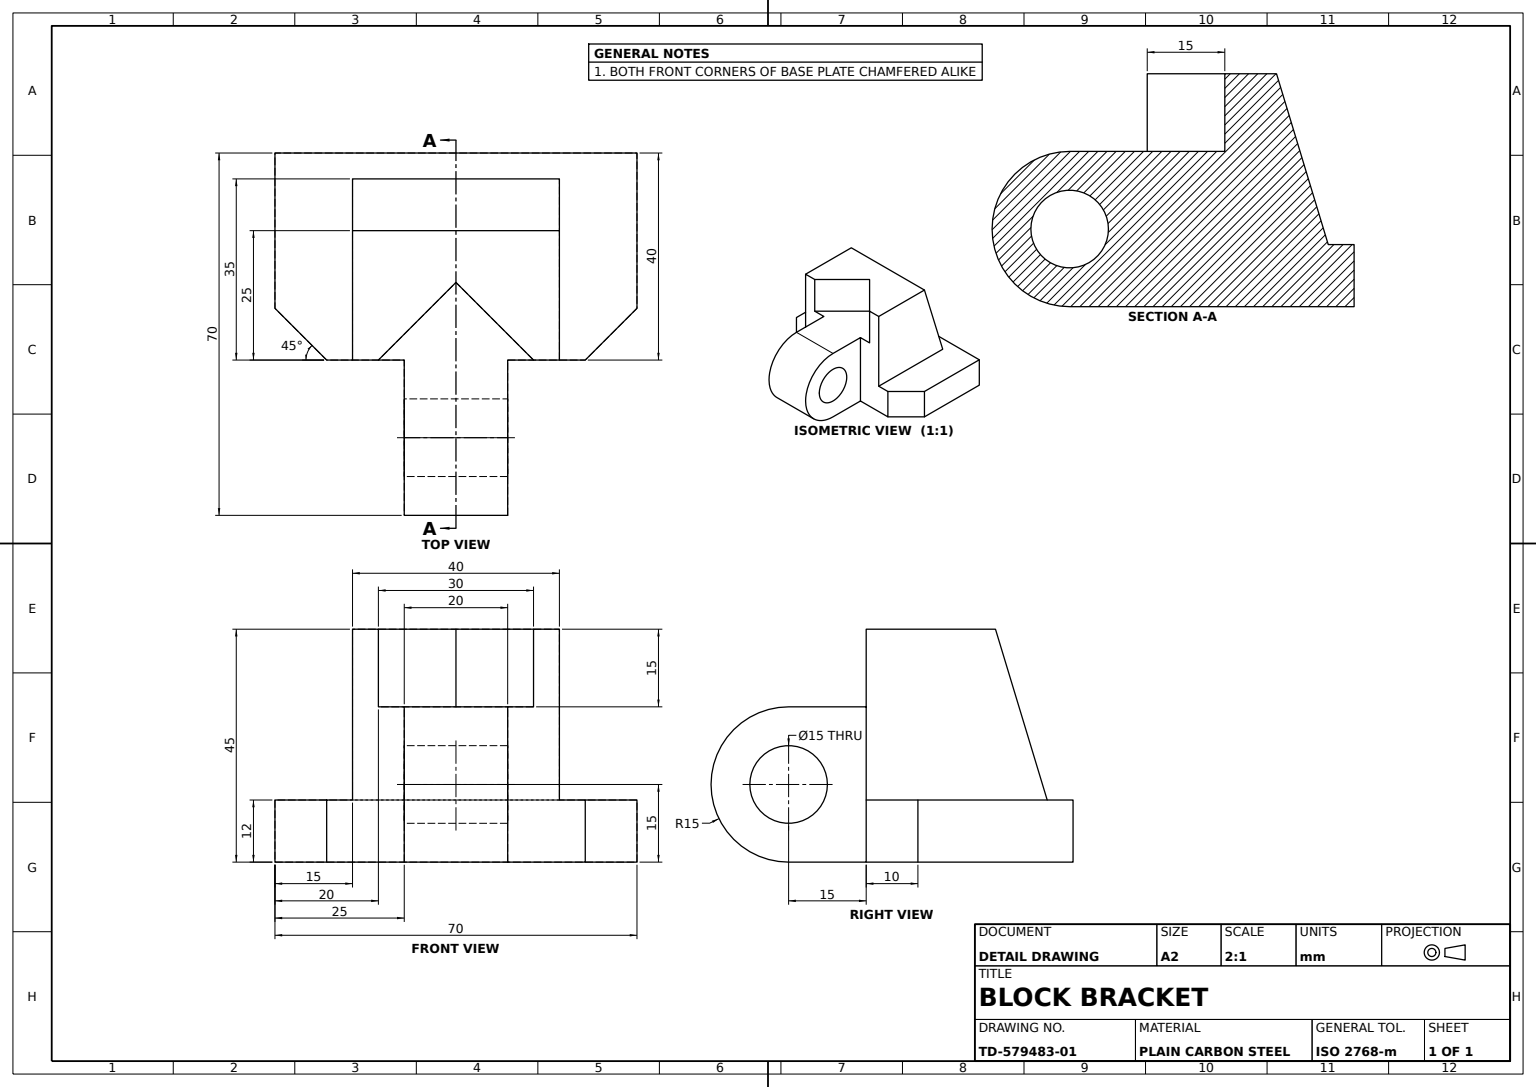
SolidWorks part; units mm, degrees
material "Plain Carbon Steel"
ref_plane "Front Plane" through (0, 0, 0) normal (0, 0, 1) x (1, 0, 0)
ref_plane "Top Plane" through (0, 0, 0) normal (0, 1, 0) x (1, 0, 0)
ref_plane "Right Plane" through (0, 0, 0) normal (1, 0, 0) x (0, 0, -1)
sketch "Base Plate Sketch" plane through (0, 0, 0) normal (0, 1, 0) x (1, 0, 0)
  line L0 (0, 0) -> (-35, 0)
  line L1 (-35, 0) -> (-35, -30)
  line L2 (-35, -30) -> (-25, -40)
  line L3 (-25, -40) -> (25, -40)
  line L4 (25, -40) -> (35, -30)
  line L5 (35, -30) -> (35, 0)
  line L6 (35, 0) -> (0, 0)
  dimension "D1" = 40
  dimension "D2" = 10
  dimension "D3" = 10
  dimension "D4" = 70
extrude "Base Plate" add sketch "Base Plate Sketch" along normal blind 12
sketch "Pedestal Bottom Profile" plane through (0, 12, 0) normal (0, 1, 0) x (1, 0, 0)
  line L0 (-20, -40) -> (-20, -5)
  line L1 (-25, -40) -> (25, -40) construction
  line L2 (-20, -5) -> (20, -5)
  line L3 (20, -5) -> (20, -40)
  line L4 (-20, -40) -> (20, -40)
  point P4 (0, -5)
  dimension "D1" = 40
  dimension "D2" = 35
ref_plane "Pedestal Top Plane" through (0, 45, 0) normal (0, 1, 0) x (1, 0, 0)
sketch "Pedestal Top Profile" plane through (0, 45, 0) normal (0, 1, 0) x (1, 0, 0)
  line L0 (20, -5) -> (20, -40) construction
  line L1 (-20, -40) -> (20, -40)
  line L2 (-20, -40) -> (-20, -15)
  line L3 (-20, -15) -> (20, -15)
  line L4 (20, -40) -> (20, -15)
  dimension "D1" = 25
loft "Tapered Pedestal" add profiles "Pedestal Top Profile", "Pedestal Bottom Profile"
sketch "Journal Boss Sketch" plane through (0, 0, 0) normal (1, 0, 0) x (0, 0, -1)
  line L0 (-40, 30) -> (-55, 30)
  line L1 (-40, 45) -> (-40, 12) construction
  line L2 (-40, 0) -> (-55, 0)
  line L3 (-40, 30) -> (-40, 0)
  arc A0 (-55, 0) -> (-55, 30) centre (-55, 15) cw
  circle A1 centre (-55, 15) radius 7.5
  point P10 (-70, 15)
  dimension "D2" = 15
  dimension "D1" = 30
  dimension "D3" = 70
extrude "Journal Boss" add sketch "Journal Boss Sketch" along normal mid plane 20
sketch "Cradle Slot Sketch" plane through (0, 45, 0) normal (0, 1, 0) x (1, 0, 0)
  line L0 (-15, -40) -> (0, -25)
  line L1 (-20, -40) -> (20, -40) construction
  line L2 (0, -25) -> (15, -40)
  line L3 (15, -40) -> (-15, -40)
  line L4 (0, -40) -> (0, -32.0009) construction
  point P4 (0, -40)
  dimension "D1" = 30
  dimension "D2" = 15
extrude "Cradle Slot 30x15" cut sketch "Cradle Slot Sketch" against normal up to surface (15 mm away) up to face at (0, 30, 47.5)
